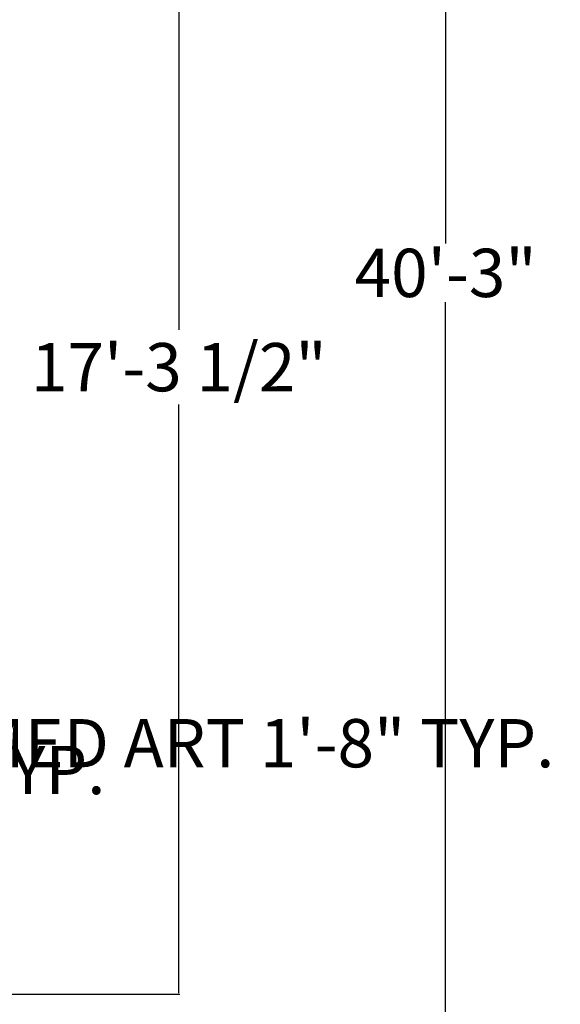
# Model space of a CAD drawing. Units: inches. Extents: x 125 to 976, y 231 to 853.
# Tile 10 of 16: x 468 to 557, y 449 to 613. Entities that reach past the tile are written whole.
import ezdxf

# ---------------------------------------------------------------- set-up
doc = ezdxf.new("R2010")
doc.units = ezdxf.units.IN
doc.header["$MEASUREMENT"] = 0
doc.layers.add('A-ANNO-DIMS', color=2, linetype='Continuous', lineweight=18)
doc.styles.get("Standard").update_dxf_attribs({"font": 'italic8.shx'})
doc.dimstyles.get("Standard").update_dxf_attribs({"dimtxt": 8, "dimasz": 0.18, "dimexe": 0.18, "dimexo": 0.0625, "dimgap": 0.09, "dimtad": 0, "dimtih": 1, "dimtoh": 1, "dimdec": 4, "dimzin": 0, "dimdsep": 46, "dimlunit": 3, "dimtxsty": 'Standard', "dimcen": 0.09, "dimclrt": 4, "dimadec": 0, "dimazin": 0, "dimtfac": 1, "dimtdec": 4, "dimtofl": 0, "dimtmove": 0, "dimatfit": 3, "dimfxl": 1, "dimtolj": 1, "dimtzin": 0, "dimarcsym": 0})

# ---------------------------------------------------------------- blocks, each defined once
blk = doc.blocks.new('*D40')
at = {"layer": 'A-ANNO-DIMS', "color": 0, "lineweight": -2, "transparency": 16777216}
for p, q in [((322.59, 494.04), (322.59, 488.07)), ((361.59, 494.04), (361.59, 488.07)), ((322.77, 488.25), (361.41, 488.25)), ((361.59, 488.25), (361.77, 488.25))]:
    blk.add_line(p, q, dxfattribs=at)
at = {"layer": 'A-ANNO-DIMS', "color": 0, "transparency": 16777216}
for points in [[(322.77, 488.28), (322.77, 488.22), (322.59, 488.25)], [(361.41, 488.28), (361.41, 488.22), (361.59, 488.25)]]:
    blk.add_solid(points, dxfattribs=at)
at = {"layer": 'Defpoints', "color": 0, "transparency": 16777216}
for p in [(322.59, 494.1), (361.59, 494.1), (361.59, 488.25)]:
    blk.add_point(p, dxfattribs=at)
at = {"layer": 'A-ANNO-DIMS', "color": 4, "transparency": 16777216, "insert": (432.52, 488.25), "char_height": 8, "attachment_point": 5}
blk.add_mtext('\\A1;RH DOOR 3\'-3" TYP.', dxfattribs=at)
blk = doc.blocks.new('*D44')
at = {"layer": 'A-ANNO-DIMS', "color": 0, "lineweight": -2, "transparency": 16777216}
for p, q in [((394.87, 489.71), (394.87, 492.87)), ((395.05, 492.69), (414.93, 492.69)), ((415.11, 489.71), (415.11, 492.87)), ((415.11, 492.69), (415.29, 492.69))]:
    blk.add_line(p, q, dxfattribs=at)
at = {"layer": 'A-ANNO-DIMS', "color": 0, "transparency": 16777216}
for points in [[(395.05, 492.72), (395.05, 492.66), (394.87, 492.69)], [(414.93, 492.72), (414.93, 492.66), (415.11, 492.69)]]:
    blk.add_solid(points, dxfattribs=at)
at = {"layer": 'Defpoints', "color": 0, "transparency": 16777216}
for p in [(415.11, 492.69), (394.87, 489.65), (415.11, 489.65)]:
    blk.add_point(p, dxfattribs=at)
at = {"layer": 'A-ANNO-DIMS', "color": 4, "transparency": 16777216, "insert": (498.42, 492.69), "char_height": 8, "attachment_point": 5}
blk.add_mtext('\\A1;FRAMED ART 1\'-8" TYP.', dxfattribs=at)
blk = doc.blocks.new('*D57')
at = {"layer": 'A-ANNO-DIMS', "color": 0, "lineweight": -2, "transparency": 16777216}
for p, q in [((567.13, 812.1), (538.31, 812.1)), ((538.49, 811.92), (538.49, 575.46)), ((538.49, 329.28), (538.49, 565.75)), ((576.13, 329.1), (538.31, 329.1))]:
    blk.add_line(p, q, dxfattribs=at)
at = {"layer": 'A-ANNO-DIMS', "color": 0, "transparency": 16777216}
for points in [[(538.46, 811.92), (538.52, 811.92), (538.49, 812.1)], [(538.46, 329.28), (538.52, 329.28), (538.49, 329.1)]]:
    blk.add_solid(points, dxfattribs=at)
at = {"layer": 'Defpoints', "color": 0, "transparency": 16777216}
for p in [(538.49, 812.1), (567.19, 812.1), (576.19, 329.1)]:
    blk.add_point(p, dxfattribs=at)
at = {"layer": 'A-ANNO-DIMS', "color": 4, "transparency": 16777216, "insert": (538.49, 570.6), "char_height": 8, "attachment_point": 5}
blk.add_mtext('\\A1;40\'-3"', dxfattribs=at)
blk = doc.blocks.new('*D64')
at = {"layer": 'A-ANNO-DIMS', "color": 0, "lineweight": -2, "transparency": 16777216}
for p, q in [((465.64, 658.83), (494.46, 658.83)), ((494.28, 658.65), (494.28, 561.16)), ((494.28, 451.31), (494.28, 548.79)), ((465.64, 451.13), (494.46, 451.13))]:
    blk.add_line(p, q, dxfattribs=at)
at = {"layer": 'A-ANNO-DIMS', "color": 0, "transparency": 16777216}
for points in [[(494.25, 658.65), (494.31, 658.65), (494.28, 658.83)], [(494.25, 451.31), (494.31, 451.31), (494.28, 451.13)]]:
    blk.add_solid(points, dxfattribs=at)
at = {"layer": 'Defpoints', "color": 0, "transparency": 16777216}
for p in [(465.58, 658.83), (494.28, 658.83), (465.58, 451.13)]:
    blk.add_point(p, dxfattribs=at)
at = {"layer": 'A-ANNO-DIMS', "color": 4, "transparency": 16777216, "insert": (494.28, 554.98), "char_height": 8, "attachment_point": 5}
blk.add_mtext('\\A1;17\'-3 1/2"', dxfattribs=at)

msp = doc.modelspace()

# ---------------------------------------------------------------- dimensions: what is measured, and where the dimension line sits
at = {"layer": 'A-ANNO-DIMS'}
for base, p1, p2, picture, middle in [((538.49287, 812.10475), (576.19287, 329.10475), (567.19287, 812.10475), '*D57', (538.49287, 570.60475)), ((494.2792, 658.82838), (465.5792, 451.12515), (465.5792, 658.82838), '*D64', (494.2792, 554.97677))]:
    dim = msp.add_linear_dim(base=base, p1=p1, p2=p2, angle=90, dimstyle='Standard', override={"dimdec": 1, "dimlfac": 1, "dimrnd": 0, "dimzin": 1, "dimdsep": 46, "dimlunit": 4, "dimfrac": 2}, dxfattribs=at)
    dim.commit()
    dim.dimension.update_dxf_attribs({"geometry": picture, "text_midpoint": middle})
for base, p1, p2, text, picture, middle in [((415.10718, 492.68858), (394.86616, 489.65243), (415.10718, 489.65243), 'FRAMED ART <> TYP.', '*D44', (498.4248, 492.68858)), ((361.58656, 488.25475), (322.58656, 494.10475), (361.58656, 494.10475), 'RH DOOR <> TYP.', '*D40', (432.52323, 488.25475))]:
    dim = msp.add_linear_dim(base=base, p1=p1, p2=p2, text=text, dimstyle='Standard', override={"dimdec": 1, "dimlfac": 1, "dimrnd": 0, "dimzin": 1, "dimdsep": 46, "dimlunit": 4, "dimfrac": 2}, dxfattribs=at)
    dim.commit()
    dim.dimension.update_dxf_attribs({"geometry": picture, "text_midpoint": middle})

doc.saveas('drawing.dxf')
